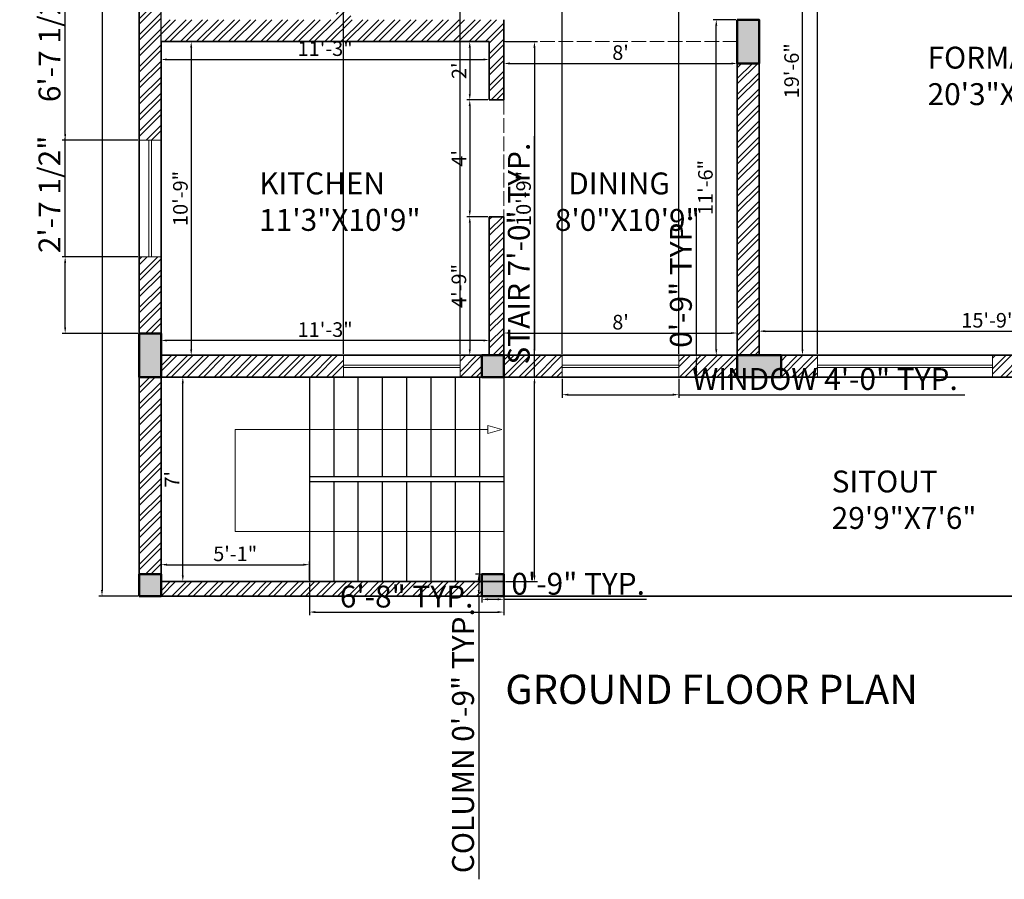
# Model space of a CAD drawing. Units: inches. Extents: x 4153 to 5577, y 785 to 1503.
# Tile 6 of 11: x 4962 to 5367, y 785 to 1138. Entities that reach past the tile are written whole.
import ezdxf

# ---------------------------------------------------------------- set-up
doc = ezdxf.new("R2010")
doc.units = ezdxf.units.IN
doc.linetypes.add('ACAD_ISO02W100', pattern=[15, 12, -3])
for name, color, linetype, lineweight in [('A-ANNO-DIMS', 2, 'Continuous', 18), ('A-ANNO-SYMB', 7, 'Continuous', 18), ('A-ANNO-TEXT', 7, 'Continuous', 35), ('A-AREA-IDEN', 7, 'Continuous', 25), ('A-COLS', 7, 'Continuous', 50), ('A-FLOR-STRS', 7, 'Continuous', 25), ('A-GLAZ', 4, 'Continuous', 18), ('A-WALL', 7, 'Continuous', 35), ('A-WALL-OVHD', 7, 'ACAD_ISO02W100', 18)]:
    doc.layers.add(name, color=color, linetype=linetype, lineweight=lineweight)
doc.layers.add('A-WALL-PATT', color=251, linetype='Continuous', lineweight=13, true_color=0x636466)
doc.styles.get("Standard").update_dxf_attribs({"font": 'arial.ttf'})
doc.dimstyles.new('ISO-25', dxfattribs={"dimtxt": 9, "dimasz": 2.5, "dimexe": 1.25, "dimexo": 0.625, "dimtad": 1, "dimlunit": 3, "dimtxsty": 'Standard', "dimcen": 2.5, "dimadec": 0, "dimazin": 0, "dimtfac": 1, "dimtmove": 0, "dimatfit": 3, "dimfxl": 1, "dimarcsym": 0})

# ---------------------------------------------------------------- blocks, each defined once
blk = doc.blocks.new('*D24')
at = {"layer": 'A-ANNO-DIMS', "color": 0, "lineweight": -2, "transparency": 16777216}
for p, q in [((5010.63, 1444.49), (4994.72, 1444.49)), ((4995.97, 1441.99), (4995.97, 903.99)), ((5010.63, 901.49), (4994.72, 901.49))]:
    blk.add_line(p, q, dxfattribs=at)
at = {"layer": 'A-ANNO-DIMS', "color": 0, "transparency": 16777216}
for points in [[(4995.55, 1441.99), (4996.38, 1441.99), (4995.97, 1444.49)], [(4995.55, 903.99), (4996.38, 903.99), (4995.97, 901.49)]]:
    blk.add_solid(points, dxfattribs=at)
at = {"layer": 'Defpoints', "color": 0, "transparency": 16777216}
for p in [(5011.25, 1444.49), (4995.97, 901.49), (5011.25, 901.49)]:
    blk.add_point(p, dxfattribs=at)
at = {"layer": 'A-ANNO-DIMS', "color": 0, "transparency": 16777216, "insert": (4990.74, 1172.99), "char_height": 9, "attachment_point": 5, "rotation": 90}
blk.add_mtext('45\'-3"', dxfattribs=at)
blk = doc.blocks.new('*D44')
at = {"layer": 'A-ANNO-DIMS', "color": 0, "lineweight": -2, "transparency": 16777216}
for p, q in [((5020.88, 1129.49), (5033.91, 1129.49)), ((5032.66, 1126.99), (5032.66, 1002.99)), ((5020.88, 1000.49), (5033.91, 1000.49))]:
    blk.add_line(p, q, dxfattribs=at)
at = {"layer": 'A-ANNO-DIMS', "color": 0, "transparency": 16777216}
for points in [[(5032.25, 1126.99), (5033.08, 1126.99), (5032.66, 1129.49)], [(5032.25, 1002.99), (5033.08, 1002.99), (5032.66, 1000.49)]]:
    blk.add_solid(points, dxfattribs=at)
at = {"layer": 'Defpoints', "color": 0, "transparency": 16777216}
for p in [(5020.25, 1129.49), (5020.25, 1000.49), (5032.66, 1000.49)]:
    blk.add_point(p, dxfattribs=at)
at = {"layer": 'A-ANNO-DIMS', "color": 0, "transparency": 16777216, "insert": (5028.97, 1064.99), "char_height": 6, "attachment_point": 5, "rotation": 90}
blk.add_mtext('10\'-9"', dxfattribs=at)
blk = doc.blocks.new('*D45')
at = {"layer": 'A-ANNO-DIMS', "color": 0, "lineweight": -2, "transparency": 16777216}
for p, q in [((5020.25, 1128.86), (5020.25, 1120.87)), ((5155.25, 1128.86), (5155.25, 1120.87)), ((5022.75, 1122.12), (5152.75, 1122.12))]:
    blk.add_line(p, q, dxfattribs=at)
at = {"layer": 'A-ANNO-DIMS', "color": 0, "transparency": 16777216}
for points in [[(5022.75, 1122.54), (5022.75, 1121.71), (5020.25, 1122.12)], [(5152.75, 1122.54), (5152.75, 1121.71), (5155.25, 1122.12)]]:
    blk.add_solid(points, dxfattribs=at)
at = {"layer": 'Defpoints', "color": 0, "transparency": 16777216}
for p in [(5020.25, 1129.49), (5155.25, 1129.49), (5155.25, 1122.12)]:
    blk.add_point(p, dxfattribs=at)
at = {"layer": 'A-ANNO-DIMS', "color": 0, "transparency": 16777216, "insert": (5087.75, 1125.81), "char_height": 6, "attachment_point": 5}
blk.add_mtext('11\'-3"', dxfattribs=at)
blk = doc.blocks.new('*D46')
at = {"layer": 'A-ANNO-DIMS', "color": 0, "lineweight": -2, "transparency": 16777216}
for p, q in [((5154.63, 1129.49), (5145.98, 1129.49)), ((5147.23, 1126.99), (5147.23, 1107.99)), ((5154.63, 1105.49), (5145.98, 1105.49))]:
    blk.add_line(p, q, dxfattribs=at)
at = {"layer": 'A-ANNO-DIMS', "color": 0, "transparency": 16777216}
for points in [[(5146.81, 1126.99), (5147.65, 1126.99), (5147.23, 1129.49)], [(5146.81, 1107.99), (5147.65, 1107.99), (5147.23, 1105.49)]]:
    blk.add_solid(points, dxfattribs=at)
at = {"layer": 'Defpoints', "color": 0, "transparency": 16777216}
for p in [(5155.25, 1129.49), (5147.23, 1105.49), (5155.25, 1105.49)]:
    blk.add_point(p, dxfattribs=at)
at = {"layer": 'A-ANNO-DIMS', "color": 0, "transparency": 16777216, "insert": (5143.59, 1117.49), "char_height": 6, "attachment_point": 5, "rotation": 90}
blk.add_mtext("2'", dxfattribs=at)
blk = doc.blocks.new('*D47')
at = {"layer": 'A-ANNO-DIMS', "color": 0, "lineweight": -2, "transparency": 16777216}
for p, q in [((5154.63, 1105.49), (5145.98, 1105.49)), ((5147.23, 1102.99), (5147.23, 1059.99)), ((5154.63, 1057.49), (5145.98, 1057.49))]:
    blk.add_line(p, q, dxfattribs=at)
at = {"layer": 'A-ANNO-DIMS', "color": 0, "transparency": 16777216}
for points in [[(5146.81, 1102.99), (5147.65, 1102.99), (5147.23, 1105.49)], [(5146.81, 1059.99), (5147.65, 1059.99), (5147.23, 1057.49)]]:
    blk.add_solid(points, dxfattribs=at)
at = {"layer": 'Defpoints', "color": 0, "transparency": 16777216}
for p in [(5155.25, 1105.49), (5147.23, 1057.49), (5155.25, 1057.49)]:
    blk.add_point(p, dxfattribs=at)
at = {"layer": 'A-ANNO-DIMS', "color": 0, "transparency": 16777216, "insert": (5143.61, 1081.49), "char_height": 6, "attachment_point": 5, "rotation": 90}
blk.add_mtext("4'", dxfattribs=at)
blk = doc.blocks.new('*D48')
at = {"layer": 'A-ANNO-DIMS', "color": 0, "lineweight": -2, "transparency": 16777216}
for p, q in [((5154.63, 1057.49), (5145.98, 1057.49)), ((5147.23, 1054.99), (5147.23, 1002.99)), ((5154.63, 1000.49), (5145.98, 1000.49))]:
    blk.add_line(p, q, dxfattribs=at)
at = {"layer": 'A-ANNO-DIMS', "color": 0, "transparency": 16777216}
for points in [[(5146.81, 1054.99), (5147.65, 1054.99), (5147.23, 1057.49)], [(5146.81, 1002.99), (5147.65, 1002.99), (5147.23, 1000.49)]]:
    blk.add_solid(points, dxfattribs=at)
at = {"layer": 'Defpoints', "color": 0, "transparency": 16777216}
for p in [(5155.25, 1057.49), (5147.23, 1000.49), (5155.25, 1000.49)]:
    blk.add_point(p, dxfattribs=at)
at = {"layer": 'A-ANNO-DIMS', "color": 0, "transparency": 16777216, "insert": (5143.54, 1028.99), "char_height": 6, "attachment_point": 5, "rotation": 90}
blk.add_mtext('4\'-9"', dxfattribs=at)
blk = doc.blocks.new('*D49')
at = {"layer": 'A-ANNO-DIMS', "color": 0, "lineweight": -2, "transparency": 16777216}
for p, q in [((5020.25, 1001.11), (5020.25, 1007.84)), ((5152.75, 1006.59), (5022.75, 1006.59)), ((5155.25, 1001.11), (5155.25, 1007.84))]:
    blk.add_line(p, q, dxfattribs=at)
at = {"layer": 'A-ANNO-DIMS', "color": 0, "transparency": 16777216}
for points in [[(5022.75, 1007), (5022.75, 1006.17), (5020.25, 1006.59)], [(5152.75, 1007), (5152.75, 1006.17), (5155.25, 1006.59)]]:
    blk.add_solid(points, dxfattribs=at)
at = {"layer": 'Defpoints', "color": 0, "transparency": 16777216}
for p in [(5020.25, 1006.59), (5020.25, 1000.49), (5155.25, 1000.49)]:
    blk.add_point(p, dxfattribs=at)
at = {"layer": 'A-ANNO-DIMS', "color": 0, "transparency": 16777216, "insert": (5087.75, 1010.28), "char_height": 6, "attachment_point": 5}
blk.add_mtext('11\'-3"', dxfattribs=at)
blk = doc.blocks.new('*D50')
at = {"layer": 'A-ANNO-DIMS', "color": 0, "lineweight": -2, "transparency": 16777216}
for p, q in [((5161.25, 1128.86), (5161.25, 1119.24)), ((5257.25, 1128.86), (5257.25, 1119.24)), ((5163.75, 1120.49), (5254.75, 1120.49))]:
    blk.add_line(p, q, dxfattribs=at)
at = {"layer": 'A-ANNO-DIMS', "color": 0, "transparency": 16777216}
for points in [[(5163.75, 1120.91), (5163.75, 1120.07), (5161.25, 1120.49)], [(5254.75, 1120.91), (5254.75, 1120.07), (5257.25, 1120.49)]]:
    blk.add_solid(points, dxfattribs=at)
at = {"layer": 'Defpoints', "color": 0, "transparency": 16777216}
for p in [(5161.25, 1129.49), (5257.25, 1129.49), (5257.25, 1120.49)]:
    blk.add_point(p, dxfattribs=at)
at = {"layer": 'A-ANNO-DIMS', "color": 0, "transparency": 16777216, "insert": (5209.25, 1124.18), "char_height": 6, "attachment_point": 5}
blk.add_mtext("8'", dxfattribs=at)
blk = doc.blocks.new('*D51')
at = {"layer": 'A-ANNO-DIMS', "color": 0, "lineweight": -2, "transparency": 16777216}
for p, q in [((5161.88, 1129.49), (5175.08, 1129.49)), ((5173.83, 1126.99), (5173.83, 1002.99)), ((5161.88, 1000.49), (5175.08, 1000.49))]:
    blk.add_line(p, q, dxfattribs=at)
at = {"layer": 'A-ANNO-DIMS', "color": 0, "transparency": 16777216}
for points in [[(5173.41, 1126.99), (5174.24, 1126.99), (5173.83, 1129.49)], [(5173.41, 1002.99), (5174.24, 1002.99), (5173.83, 1000.49)]]:
    blk.add_solid(points, dxfattribs=at)
at = {"layer": 'Defpoints', "color": 0, "transparency": 16777216}
for p in [(5161.25, 1129.49), (5161.25, 1000.49), (5173.83, 1000.49)]:
    blk.add_point(p, dxfattribs=at)
at = {"layer": 'A-ANNO-DIMS', "color": 0, "transparency": 16777216, "insert": (5170.14, 1064.99), "char_height": 6, "attachment_point": 5, "rotation": 90}
blk.add_mtext('10\'-9"', dxfattribs=at)
blk = doc.blocks.new('*D52')
at = {"layer": 'A-ANNO-DIMS', "color": 0, "lineweight": -2, "transparency": 16777216}
for p, q in [((5161.25, 1001.11), (5161.25, 1010.89)), ((5163.75, 1009.64), (5254.75, 1009.64)), ((5257.25, 1001.11), (5257.25, 1010.89))]:
    blk.add_line(p, q, dxfattribs=at)
at = {"layer": 'A-ANNO-DIMS', "color": 0, "transparency": 16777216}
for points in [[(5163.75, 1010.05), (5163.75, 1009.22), (5161.25, 1009.64)], [(5254.75, 1010.05), (5254.75, 1009.22), (5257.25, 1009.64)]]:
    blk.add_solid(points, dxfattribs=at)
at = {"layer": 'Defpoints', "color": 0, "transparency": 16777216}
for p in [(5257.25, 1009.64), (5161.25, 1000.49), (5257.25, 1000.49)]:
    blk.add_point(p, dxfattribs=at)
at = {"layer": 'A-ANNO-DIMS', "color": 0, "transparency": 16777216, "insert": (5209.25, 1013.33), "char_height": 6, "attachment_point": 5}
blk.add_mtext("8'", dxfattribs=at)
blk = doc.blocks.new('*D53')
at = {"layer": 'A-ANNO-DIMS', "color": 0, "lineweight": -2, "transparency": 16777216}
for p, q in [((5256.63, 1138.49), (5247.37, 1138.49)), ((5248.62, 1002.99), (5248.62, 1135.99)), ((5256.63, 1000.49), (5247.37, 1000.49))]:
    blk.add_line(p, q, dxfattribs=at)
at = {"layer": 'A-ANNO-DIMS', "color": 0, "transparency": 16777216}
for points in [[(5248.2, 1135.99), (5249.04, 1135.99), (5248.62, 1138.49)], [(5248.2, 1002.99), (5249.04, 1002.99), (5248.62, 1000.49)]]:
    blk.add_solid(points, dxfattribs=at)
at = {"layer": 'Defpoints', "color": 0, "transparency": 16777216}
for p in [(5248.62, 1138.49), (5257.25, 1138.49), (5257.25, 1000.49)]:
    blk.add_point(p, dxfattribs=at)
at = {"layer": 'A-ANNO-DIMS', "color": 0, "transparency": 16777216, "insert": (5244.93, 1069.49), "char_height": 6, "attachment_point": 5, "rotation": 90}
blk.add_mtext('11\'-6"', dxfattribs=at)
blk = doc.blocks.new('*D54')
at = {"layer": 'A-ANNO-DIMS', "color": 0, "lineweight": -2, "transparency": 16777216}
for p, q in [((5266.88, 1234.49), (5285.33, 1234.49)), ((5284.08, 1002.99), (5284.08, 1231.99)), ((5266.88, 1000.49), (5285.33, 1000.49))]:
    blk.add_line(p, q, dxfattribs=at)
at = {"layer": 'A-ANNO-DIMS', "color": 0, "transparency": 16777216}
for points in [[(5283.66, 1231.99), (5284.49, 1231.99), (5284.08, 1234.49)], [(5283.66, 1002.99), (5284.49, 1002.99), (5284.08, 1000.49)]]:
    blk.add_solid(points, dxfattribs=at)
at = {"layer": 'Defpoints', "color": 0, "transparency": 16777216}
for p in [(5266.25, 1234.49), (5284.08, 1234.49), (5266.25, 1000.49)]:
    blk.add_point(p, dxfattribs=at)
at = {"layer": 'A-ANNO-DIMS', "color": 0, "transparency": 16777216, "insert": (5280.39, 1117.49), "char_height": 6, "attachment_point": 5, "rotation": 90}
blk.add_mtext('19\'-6"', dxfattribs=at)
blk = doc.blocks.new('*D55')
at = {"layer": 'A-ANNO-DIMS', "color": 0, "lineweight": -2, "transparency": 16777216}
for p, q in [((5266.25, 1001.11), (5266.25, 1011.66)), ((5268.75, 1010.41), (5452.75, 1010.41)), ((5455.25, 1001.11), (5455.25, 1011.66))]:
    blk.add_line(p, q, dxfattribs=at)
at = {"layer": 'A-ANNO-DIMS', "color": 0, "transparency": 16777216}
for points in [[(5268.75, 1010.82), (5268.75, 1009.99), (5266.25, 1010.41)], [(5452.75, 1010.82), (5452.75, 1009.99), (5455.25, 1010.41)]]:
    blk.add_solid(points, dxfattribs=at)
at = {"layer": 'Defpoints', "color": 0, "transparency": 16777216}
for p in [(5455.25, 1010.41), (5266.25, 1000.49), (5455.25, 1000.49)]:
    blk.add_point(p, dxfattribs=at)
at = {"layer": 'A-ANNO-DIMS', "color": 0, "transparency": 16777216, "insert": (5360.75, 1014.1), "char_height": 6, "attachment_point": 5}
blk.add_mtext('15\'-9"', dxfattribs=at)
blk = doc.blocks.new('*D87')
at = {"layer": 'A-ANNO-DIMS', "color": 0, "lineweight": -2, "transparency": 16777216}
for p, q in [((5020.88, 991.49), (5030.45, 991.49)), ((5029.2, 909.99), (5029.2, 988.99)), ((5020.88, 907.49), (5030.45, 907.49))]:
    blk.add_line(p, q, dxfattribs=at)
at = {"layer": 'A-ANNO-DIMS', "color": 0, "transparency": 16777216}
for points in [[(5028.78, 988.99), (5029.61, 988.99), (5029.2, 991.49)], [(5028.78, 909.99), (5029.61, 909.99), (5029.2, 907.49)]]:
    blk.add_solid(points, dxfattribs=at)
at = {"layer": 'Defpoints', "color": 0, "transparency": 16777216}
for p in [(5020.25, 991.49), (5029.2, 991.49), (5020.25, 907.49)]:
    blk.add_point(p, dxfattribs=at)
at = {"layer": 'A-ANNO-DIMS', "color": 0, "transparency": 16777216, "insert": (5025.57, 949.49), "char_height": 6, "attachment_point": 5, "rotation": 90}
blk.add_mtext("7'", dxfattribs=at)
blk = doc.blocks.new('*D88')
at = {"layer": 'A-ANNO-DIMS', "color": 0, "lineweight": -2, "transparency": 16777216}
for p, q in [((5020.25, 908.11), (5020.25, 915.63)), ((5081.25, 908.11), (5081.25, 915.63)), ((5022.75, 914.38), (5078.75, 914.38))]:
    blk.add_line(p, q, dxfattribs=at)
at = {"layer": 'A-ANNO-DIMS', "color": 0, "transparency": 16777216}
for points in [[(5022.75, 914.8), (5022.75, 913.97), (5020.25, 914.38)], [(5078.75, 914.8), (5078.75, 913.97), (5081.25, 914.38)]]:
    blk.add_solid(points, dxfattribs=at)
at = {"layer": 'Defpoints', "color": 0, "transparency": 16777216}
for p in [(5081.25, 914.38), (5020.25, 907.49), (5081.25, 907.49)]:
    blk.add_point(p, dxfattribs=at)
at = {"layer": 'A-ANNO-DIMS', "color": 0, "transparency": 16777216, "insert": (5050.75, 918.07), "char_height": 6, "attachment_point": 5}
blk.add_mtext('5\'-1"', dxfattribs=at)
blk = doc.blocks.new('WINDOW-48IN')
for p, q in [((0, 9), (0, 0)), ((48, 9), (48, 0)), ((0, 5), (48, 5)), ((0, 4), (48, 4))]:
    blk.add_line(p, q)
blk = doc.blocks.new('WINDOW-72IN')
for p, q in [((0, 9), (0, 0)), ((72, 9), (72, 0)), ((0, 5), (72, 5)), ((0, 4), (72, 4))]:
    blk.add_line(p, q)
blk = doc.blocks.new('COL-9X18IN')
at = {"transparency": 33554687}
h = blk.add_hatch(color=256, dxfattribs=at)
h.dxf.hatch_style = 1
h.paths.add_polyline_path([(9, 18), (0, 18), (0, 0), (9, 0)])
blk.add_lwpolyline([(0, 18), (9, 18), (9, 0), (0, 0)], close=True)
blk = doc.blocks.new('COL-9X9IN')
at = {"transparency": 33554687}
h = blk.add_hatch(color=256, dxfattribs=at)
h.dxf.hatch_style = 1
h.paths.add_polyline_path([(9, 0), (9, 9), (0, 9), (0, 0)])
blk.add_lwpolyline([(0, 9), (9, 9), (9, 0), (0, 0)], close=True)
blk = doc.blocks.new('SITOUT-RETURN-STAIR')
at = {"ltscale": 0.5}
for p, q in [((0, 84), (0, 41)), ((10, 84), (10, 43)), ((20, 84), (20, 43)), ((30, 84), (30, 43)), ((40, 84), (40, 43)), ((50, 84), (50, 43)), ((60, 84), (60, 43)), ((70, 84), (70, 43)), ((80, 84), (80, 41))]:
    blk.add_line(p, q, dxfattribs=at)
for p, q in [((80, 43), (0, 43)), ((80, 41), (0, 41)), ((0, 41), (0, 0)), ((10, 41), (10, 0)), ((20, 41), (20, 0)), ((30, 41), (30, 0)), ((40, 41), (40, 0)), ((50, 41), (50, 0)), ((60, 41), (60, 0)), ((70, 41), (70, 0)), ((80, 41), (80, 0))]:
    blk.add_line(p, q)
blk = doc.blocks.new('STAIR-DIRECTION-RETURN')
at = {"ltscale": 0.5}
for p, q in [((103.89, 42), (0, 42)), ((0, 0), (0, 42)), ((110.5, 0), (0, 0))]:
    blk.add_line(p, q, dxfattribs=at)
blk.add_lwpolyline([(109.65, 42), (103.89, 43.63), (103.89, 40.37)], close=True)
blk = doc.blocks.new('*D100')
at = {"layer": 'A-ANNO-DIMS', "color": 0, "lineweight": -2, "transparency": 16777216}
for p, q in [((5151.63, 910.49), (5149.65, 910.49)), ((5150.9, 907.99), (5150.9, 903.99)), ((5151.63, 901.49), (5149.65, 901.49)), ((5150.9, 901.49), (5150.9, 785.01))]:
    blk.add_line(p, q, dxfattribs=at)
at = {"layer": 'A-ANNO-DIMS', "color": 0, "transparency": 16777216}
for points in [[(5150.49, 907.99), (5151.32, 907.99), (5150.9, 910.49)], [(5150.49, 903.99), (5151.32, 903.99), (5150.9, 901.49)]]:
    blk.add_solid(points, dxfattribs=at)
at = {"layer": 'Defpoints', "color": 0, "transparency": 16777216}
for p in [(5152.25, 910.49), (5150.9, 901.49), (5152.25, 901.49)]:
    blk.add_point(p, dxfattribs=at)
at = {"layer": 'A-ANNO-DIMS', "color": 0, "transparency": 16777216, "insert": (5145.62, 842), "char_height": 9, "attachment_point": 5, "rotation": 90}
blk.add_mtext('COLUMN 0\'-9" TYP.', dxfattribs=at)
blk = doc.blocks.new('*D101')
at = {"layer": 'A-ANNO-DIMS', "color": 0, "lineweight": -2, "transparency": 16777216}
for p, q in [((5152.25, 900.86), (5152.25, 898.89)), ((5154.75, 900.14), (5158.75, 900.14)), ((5161.25, 900.86), (5161.25, 898.89)), ((5161.25, 900.14), (5219.86, 900.14))]:
    blk.add_line(p, q, dxfattribs=at)
at = {"layer": 'A-ANNO-DIMS', "color": 0, "transparency": 16777216}
for points in [[(5154.75, 900.56), (5154.75, 899.72), (5152.25, 900.14)], [(5158.75, 900.56), (5158.75, 899.72), (5161.25, 900.14)]]:
    blk.add_solid(points, dxfattribs=at)
at = {"layer": 'Defpoints', "color": 0, "transparency": 16777216}
for p in [(5152.25, 901.49), (5161.25, 901.49), (5161.25, 900.14)]:
    blk.add_point(p, dxfattribs=at)
at = {"layer": 'A-ANNO-DIMS', "color": 0, "transparency": 16777216, "insert": (5191.81, 905.36), "char_height": 9, "attachment_point": 5}
blk.add_mtext('0\'-9" TYP.', dxfattribs=at)
blk = doc.blocks.new('*D102')
at = {"layer": 'A-ANNO-DIMS', "color": 0, "lineweight": -2, "transparency": 16777216}
for p, q in [((5185.25, 990.86), (5185.25, 983.04)), ((5233.25, 990.86), (5233.25, 983.04)), ((5187.75, 984.29), (5230.75, 984.29)), ((5233.25, 984.29), (5350.89, 984.29))]:
    blk.add_line(p, q, dxfattribs=at)
at = {"layer": 'A-ANNO-DIMS', "color": 0, "transparency": 16777216}
for points in [[(5187.75, 984.71), (5187.75, 983.87), (5185.25, 984.29)], [(5230.75, 984.71), (5230.75, 983.87), (5233.25, 984.29)]]:
    blk.add_solid(points, dxfattribs=at)
at = {"layer": 'Defpoints', "color": 0, "transparency": 16777216}
for p in [(5185.25, 991.49), (5233.25, 991.49), (5233.25, 984.29)]:
    blk.add_point(p, dxfattribs=at)
at = {"layer": 'A-ANNO-DIMS', "color": 0, "transparency": 16777216, "insert": (5293.32, 989.57), "char_height": 9, "attachment_point": 5}
blk.add_mtext('WINDOW 4\'-0" TYP.', dxfattribs=at)
blk = doc.blocks.new('*D103')
at = {"layer": 'A-ANNO-DIMS', "color": 0, "lineweight": -2, "transparency": 16777216}
for p, q in [((5240.45, 1000.49), (5240.45, 1059.1)), ((5233.88, 1000.49), (5241.7, 1000.49)), ((5240.45, 993.99), (5240.45, 997.99)), ((5233.88, 991.49), (5241.7, 991.49))]:
    blk.add_line(p, q, dxfattribs=at)
at = {"layer": 'A-ANNO-DIMS', "color": 0, "transparency": 16777216}
for points in [[(5240.04, 997.99), (5240.87, 997.99), (5240.45, 1000.49)], [(5240.04, 993.99), (5240.87, 993.99), (5240.45, 991.49)]]:
    blk.add_solid(points, dxfattribs=at)
at = {"layer": 'Defpoints', "color": 0, "transparency": 16777216}
for p in [(5233.25, 1000.49), (5240.45, 1000.49), (5233.25, 991.49)]:
    blk.add_point(p, dxfattribs=at)
at = {"layer": 'A-ANNO-DIMS', "color": 0, "transparency": 16777216, "insert": (5235.23, 1031.04), "char_height": 9, "attachment_point": 5, "rotation": 90}
blk.add_mtext('0\'-9" TYP.', dxfattribs=at)
blk = doc.blocks.new('*D140')
at = {"layer": 'A-ANNO-DIMS', "color": 0, "lineweight": -2, "transparency": 16777216}
for p, q in [((5173.85, 991.49), (5173.85, 1090.57)), ((5161.88, 991.49), (5175.1, 991.49)), ((5173.85, 909.99), (5173.85, 988.99)), ((5161.88, 907.49), (5175.1, 907.49))]:
    blk.add_line(p, q, dxfattribs=at)
at = {"layer": 'A-ANNO-DIMS', "color": 0, "transparency": 16777216}
for points in [[(5173.44, 988.99), (5174.27, 988.99), (5173.85, 991.49)], [(5173.44, 909.99), (5174.27, 909.99), (5173.85, 907.49)]]:
    blk.add_solid(points, dxfattribs=at)
at = {"layer": 'Defpoints', "color": 0, "transparency": 16777216}
for p in [(5161.25, 991.49), (5173.85, 991.49), (5161.25, 907.49)]:
    blk.add_point(p, dxfattribs=at)
at = {"layer": 'A-ANNO-DIMS', "color": 0, "transparency": 16777216, "insert": (5168.58, 1042.28), "char_height": 9, "attachment_point": 5, "rotation": 90}
blk.add_mtext('STAIR 7\'-0" TYP.', dxfattribs=at)
blk = doc.blocks.new('*D141')
at = {"layer": 'A-ANNO-DIMS', "color": 0, "lineweight": -2, "transparency": 16777216}
for p, q in [((5081.25, 906.86), (5081.25, 893.64)), ((5161.25, 906.86), (5161.25, 893.64)), ((5083.75, 894.89), (5158.75, 894.89))]:
    blk.add_line(p, q, dxfattribs=at)
at = {"layer": 'A-ANNO-DIMS', "color": 0, "transparency": 16777216}
for points in [[(5083.75, 895.31), (5083.75, 894.47), (5081.25, 894.89)], [(5158.75, 895.31), (5158.75, 894.47), (5161.25, 894.89)]]:
    blk.add_solid(points, dxfattribs=at)
at = {"layer": 'Defpoints', "color": 0, "transparency": 16777216}
for p in [(5081.25, 907.49), (5161.25, 907.49), (5161.25, 894.89)]:
    blk.add_point(p, dxfattribs=at)
at = {"layer": 'A-ANNO-DIMS', "color": 0, "transparency": 16777216, "insert": (5121.25, 900.11), "char_height": 9, "attachment_point": 5}
blk.add_mtext('6\'-8" TYP.', dxfattribs=at)
blk = doc.blocks.new('*D150')
at = {"layer": 'A-ANNO-DIMS', "color": 0, "lineweight": -2, "transparency": 16777216}
for p, q in [((4980.8, 1040.99), (4980.8, 1089.79)), ((5010.63, 1040.99), (4979.55, 1040.99)), ((4980.8, 1011.99), (4980.8, 1038.49)), ((5010.63, 1009.49), (4979.55, 1009.49))]:
    blk.add_line(p, q, dxfattribs=at)
at = {"layer": 'A-ANNO-DIMS', "color": 0, "transparency": 16777216}
for points in [[(4980.39, 1038.49), (4981.22, 1038.49), (4980.8, 1040.99)], [(4980.39, 1011.99), (4981.22, 1011.99), (4980.8, 1009.49)]]:
    blk.add_solid(points, dxfattribs=at)
at = {"layer": 'Defpoints', "color": 0, "transparency": 16777216}
for p in [(4980.8, 1040.99), (5011.25, 1040.99), (5011.25, 1009.49)]:
    blk.add_point(p, dxfattribs=at)
at = {"layer": 'A-ANNO-DIMS', "color": 0, "transparency": 16777216, "insert": (4975.53, 1066.64), "char_height": 9, "attachment_point": 5, "rotation": 90}
blk.add_mtext('2\'-7 1/2"', dxfattribs=at)
blk = doc.blocks.new('*D151')
at = {"layer": 'A-ANNO-DIMS', "color": 0, "lineweight": -2, "transparency": 16777216}
for p, q in [((5010.63, 1168.49), (4979.55, 1168.49)), ((4980.8, 1091.49), (4980.8, 1165.99)), ((5010.63, 1088.99), (4979.55, 1088.99))]:
    blk.add_line(p, q, dxfattribs=at)
at = {"layer": 'A-ANNO-DIMS', "color": 0, "transparency": 16777216}
for points in [[(4980.39, 1165.99), (4981.22, 1165.99), (4980.8, 1168.49)], [(4980.39, 1091.49), (4981.22, 1091.49), (4980.8, 1088.99)]]:
    blk.add_solid(points, dxfattribs=at)
at = {"layer": 'Defpoints', "color": 0, "transparency": 16777216}
for p in [(4980.8, 1168.49), (5011.25, 1168.49), (5011.25, 1088.99)]:
    blk.add_point(p, dxfattribs=at)
at = {"layer": 'A-ANNO-DIMS', "color": 0, "transparency": 16777216, "insert": (4975.53, 1128.74), "char_height": 9, "attachment_point": 5, "rotation": 90}
blk.add_mtext('6\'-7 1/2"', dxfattribs=at)
blk = doc.blocks.new('*D156')
at = {"layer": 'A-ANNO-DIMS', "color": 0, "lineweight": -2, "transparency": 16777216}
for p, q in [((5020.25, 1001.11), (5020.25, 1476.19)), ((5022.75, 1474.94), (5092.75, 1474.94)), ((5095.25, 1001.11), (5095.25, 1476.19))]:
    blk.add_line(p, q, dxfattribs=at)
at = {"layer": 'A-ANNO-DIMS', "color": 0, "transparency": 16777216}
for points in [[(5022.75, 1475.36), (5022.75, 1474.52), (5020.25, 1474.94)], [(5092.75, 1475.36), (5092.75, 1474.52), (5095.25, 1474.94)]]:
    blk.add_solid(points, dxfattribs=at)
at = {"layer": 'Defpoints', "color": 0, "transparency": 16777216}
for p in [(5095.25, 1474.94), (5020.25, 1000.49), (5095.25, 1000.49)]:
    blk.add_point(p, dxfattribs=at)
at = {"layer": 'A-ANNO-DIMS', "color": 0, "transparency": 16777216, "insert": (5057.75, 1480.16), "char_height": 9, "attachment_point": 5}
blk.add_mtext('6\'-3"', dxfattribs=at)
blk = doc.blocks.new('*D157')
at = {"layer": 'A-ANNO-DIMS', "color": 0, "lineweight": -2, "transparency": 16777216}
for p, q in [((5143.25, 1001.11), (5143.25, 1476.19)), ((5145.75, 1474.94), (5182.75, 1474.94)), ((5185.25, 1001.11), (5185.25, 1476.19))]:
    blk.add_line(p, q, dxfattribs=at)
at = {"layer": 'A-ANNO-DIMS', "color": 0, "transparency": 16777216}
for points in [[(5145.75, 1475.36), (5145.75, 1474.52), (5143.25, 1474.94)], [(5182.75, 1475.36), (5182.75, 1474.52), (5185.25, 1474.94)]]:
    blk.add_solid(points, dxfattribs=at)
at = {"layer": 'Defpoints', "color": 0, "transparency": 16777216}
for p in [(5185.25, 1474.94), (5143.25, 1000.49), (5185.25, 1000.49)]:
    blk.add_point(p, dxfattribs=at)
at = {"layer": 'A-ANNO-DIMS', "color": 0, "transparency": 16777216, "insert": (5164.25, 1480.16), "char_height": 9, "attachment_point": 5}
blk.add_mtext('3\'-6"', dxfattribs=at)
blk = doc.blocks.new('*D158')
at = {"layer": 'A-ANNO-DIMS', "color": 0, "lineweight": -2, "transparency": 16777216}
for p, q in [((5233.25, 1001.11), (5233.25, 1476.19)), ((5235.75, 1474.94), (5287.75, 1474.94)), ((5290.25, 1001.11), (5290.25, 1476.19))]:
    blk.add_line(p, q, dxfattribs=at)
at = {"layer": 'A-ANNO-DIMS', "color": 0, "transparency": 16777216}
for points in [[(5235.75, 1475.36), (5235.75, 1474.52), (5233.25, 1474.94)], [(5287.75, 1475.36), (5287.75, 1474.52), (5290.25, 1474.94)]]:
    blk.add_solid(points, dxfattribs=at)
at = {"layer": 'Defpoints', "color": 0, "transparency": 16777216}
for p in [(5290.25, 1474.94), (5233.25, 1000.49), (5290.25, 1000.49)]:
    blk.add_point(p, dxfattribs=at)
at = {"layer": 'A-ANNO-DIMS', "color": 0, "transparency": 16777216, "insert": (5261.75, 1480.16), "char_height": 9, "attachment_point": 5}
blk.add_mtext('4\'-9"', dxfattribs=at)

msp = doc.modelspace()

# ---------------------------------------------------------------- hatches: boundary and pattern name
at = {"layer": 'A-WALL-PATT', "transparency": 33554687}
h = msp.add_hatch(dxfattribs=at)
h.set_pattern_fill('ANSI32', color=256, scale=0.49)
h.set_pattern_definition([(45, (816.3263, 0), (-3.300244, 3.300244), []), (45, (818.5265, 0), (-3.300244, 3.300244), [])])
h.paths.add_polyline_path([(5011.254, 1088.988), (5020.254, 1088.988), (5020.254, 1129.488), (5155.254, 1129.488), (5155.254, 1105.488), (5161.254, 1105.488), (5161.254, 1138.488), (5098.254, 1138.488), (5098.254, 1234.488), (5113.254, 1234.488), (5113.254, 1243.488), (5086.254, 1243.488), (5086.254, 1234.488), (5092.254, 1234.488), (5092.254, 1138.488), (5020.254, 1138.488), (5020.254, 1168.488), (5011.254, 1168.488)])
h.paths.add_polyline_path([(5011.254, 1009.488), (5020.254, 1009.488), (5020.254, 1040.988), (5011.254, 1040.988)])
h.paths.add_polyline_path([(5095.254, 991.488), (5095.254, 1000.488), (5020.254, 1000.488), (5020.254, 991.488)])
h.paths.add_polyline_path([(5011.254, 910.488), (5020.254, 910.488), (5020.254, 991.488), (5011.254, 991.488)])
h.paths.add_polyline_path([(5152.254, 901.488), (5152.254, 907.488), (5020.254, 907.488), (5020.254, 901.488)])
h.paths.add_polyline_path([(5161.254, 1057.488), (5155.254, 1057.488), (5155.254, 1000.488), (5161.254, 1000.488)])
h.paths.add_polyline_path([(5143.254, 991.488), (5152.254, 991.488), (5152.254, 1000.488), (5143.254, 1000.488)])
h.paths.add_polyline_path([(5161.254, 1000.488), (5161.254, 991.488), (5185.254, 991.488), (5185.254, 1000.488)])
h.paths.add_polyline_path([(5257.254, 991.488), (5257.254, 1000.488), (5233.254, 1000.488), (5233.254, 991.488)])
h.paths.add_polyline_path([(5266.254, 1120.488), (5257.254, 1120.488), (5257.254, 1000.488), (5266.254, 1000.488)])
h.paths.add_polyline_path([(5290.254, 991.488), (5290.254, 1000.488), (5275.254, 1000.488), (5275.254, 991.488)])
h.paths.add_polyline_path([(5362.254, 1000.488), (5362.254, 991.488), (5455.254, 991.488), (5455.254, 1000.488)])
h.paths.add_polyline_path([(5509.254, 1009.488), (5518.254, 1009.488), (5518.254, 1036.488), (5509.254, 1036.488)])
h.paths.add_polyline_path([(5503.254, 1000.488), (5503.254, 991.488), (5509.254, 991.488), (5509.254, 1000.488)])
h.paths.add_polyline_path([(5518.254, 1132.488), (5509.254, 1132.488), (5509.254, 1108.488), (5518.254, 1108.488)])
h.paths.add_polyline_path([(5509.254, 1204.488), (5518.254, 1204.488), (5518.254, 1225.488), (5509.254, 1225.488)])
h.paths.add_polyline_path([(5467.254, 1234.488), (5467.254, 1243.488), (5377.254, 1243.488), (5377.254, 1265.228), (5377.254, 1381.488), (5467.254, 1381.488), (5467.254, 1393.488), (5461.254, 1393.488), (5461.254, 1387.488), (5377.254, 1387.488), (5377.254, 1435.488), (5368.254, 1435.488), (5368.254, 1354.488), (5347.254, 1354.488), (5347.254, 1348.488), (5368.254, 1348.488), (5368.254, 1309.488), (5302.254, 1309.488), (5302.254, 1234.488), (5321.754, 1234.488), (5321.754, 1243.488), (5311.254, 1243.488), (5311.254, 1303.488), (5368.254, 1303.488), (5368.254, 1243.488), (5357.754, 1243.488), (5357.754, 1234.488)])
h.paths.add_polyline_path([(5509.254, 1357.488), (5518.254, 1357.488), (5518.254, 1426.488), (5509.254, 1426.488)])
h.paths.add_polyline_path([(5509.254, 1243.488), (5518.254, 1243.488), (5518.254, 1309.488), (5509.254, 1309.488)])
h.paths.add_polyline_path([(5509.254, 1435.488), (5509.254, 1444.488), (5425.254, 1444.488), (5425.254, 1435.488), (5461.254, 1435.488), (5461.254, 1423.488), (5467.254, 1423.488), (5467.254, 1435.488)])
h.paths.add_polyline_path([(5302.254, 1435.488), (5302.254, 1348.488), (5317.254, 1348.488), (5317.254, 1354.488), (5311.254, 1354.488), (5311.254, 1435.488), (5314.254, 1435.488), (5314.254, 1444.488), (5296.254, 1444.488), (5296.254, 1435.488)])
h.paths.add_polyline_path([(5368.254, 1444.488), (5362.254, 1444.488), (5362.254, 1435.488), (5368.254, 1435.488)])
h.paths.add_polyline_path([(5389.254, 1444.488), (5386.254, 1444.488), (5386.254, 1435.488), (5389.254, 1435.488)])
h.paths.add_polyline_path([(5248.254, 1435.488), (5248.254, 1444.488), (5173.254, 1444.488), (5173.254, 1435.488)])
h.paths.add_polyline_path([(5101.254, 1435.488), (5101.254, 1444.488), (5020.254, 1444.488), (5020.254, 1435.488)])
h.paths.add_polyline_path([(5011.254, 1293.488), (5020.254, 1293.488), (5020.254, 1295.242), (5020.254, 1426.488), (5011.254, 1426.488)])
h.paths.add_polyline_path([(5155.254, 1243.488), (5149.254, 1243.488), (5149.254, 1234.488), (5248.254, 1234.488), (5248.254, 1243.488), (5164.254, 1243.488), (5164.254, 1435.488), (5155.254, 1435.488)])
h.paths.add_polyline_path([(5020.254, 1243.488), (5020.254, 1234.488), (5056.254, 1234.488), (5056.254, 1243.488)], flags=17)
h.paths.add_polyline_path([(5020.254, 1225.488), (5011.254, 1225.488), (5011.254, 1198.488), (5020.254, 1198.488)], flags=17)

# ---------------------------------------------------------------- linework, layer by layer
at = {"layer": 'A-WALL'}
for p, q in [((5011.254, 901.488), (5011.254, 1444.488)), ((5161.254, 1105.488), (5161.254, 1138.488)), ((5257.254, 1000.488), (5257.254, 1138.488)), ((5266.254, 1000.488), (5266.254, 1138.488)), ((5020.254, 1129.488), (5155.254, 1129.488)), ((5020.254, 1000.488), (5020.254, 1129.488)), ((5155.254, 1105.488), (5155.254, 1129.488)), ((5155.254, 1105.488), (5161.254, 1105.488)), ((5155.254, 1000.488), (5155.254, 1057.488)), ((5155.254, 1057.488), (5161.254, 1057.488)), ((5161.254, 1000.488), (5161.254, 1057.488)), ((5020.254, 1000.488), (5155.254, 1000.488)), ((5161.254, 1000.488), (5257.254, 1000.488)), ((5266.254, 1000.488), (5455.254, 1000.488)), ((5020.254, 991.488), (5455.254, 991.488)), ((5020.254, 907.488), (5020.254, 991.488)), ((5161.254, 907.488), (5020.254, 907.488)), ((5518.254, 901.488), (5011.254, 901.488))]:
    msp.add_line(p, q, dxfattribs=at)
at = {"layer": 'A-WALL-OVHD', "ltscale": 0.5}
for p, q in [((5161.254, 1129.488), (5257.254, 1129.488)), ((5161.254, 1105.488), (5161.254, 1057.488))]:
    msp.add_line(p, q, dxfattribs=at)

# ---------------------------------------------------------------- block references
at = {"layer": 'A-ANNO-SYMB'}
msp.add_blockref('STAIR-DIRECTION-RETURN', (5050.754, 927.988), dxfattribs=at)
at = {"layer": 'A-COLS'}
for p in [(5257.254, 1120.488), (5011.254, 991.488)]:
    msp.add_blockref('COL-9X18IN', p, dxfattribs=at)
for name, p, rotation in [('COL-9X9IN', (5152.254, 1000.488), 270.0000000000087), ('COL-9X18IN', (5257.254, 1000.488), 270.0000000000049), ('COL-9X9IN', (5011.254, 910.488), 270.0000000000065), ('COL-9X9IN', (5152.254, 910.488), 270.0000000000058)]:
    msp.add_blockref(name, p, dxfattribs=dict(at, rotation=rotation))
at = {"layer": 'A-FLOR-STRS'}
msp.add_blockref('SITOUT-RETURN-STAIR', (5081.254, 907.488), dxfattribs=at)
at = {"layer": 'A-GLAZ', "rotation": 269.9999999999995}
msp.add_blockref('WINDOW-48IN', (5011.254, 1088.988), dxfattribs=at)
at = {"layer": 'A-GLAZ'}
for name, p in [('WINDOW-48IN', (5095.254, 991.488)), ('WINDOW-48IN', (5185.254, 991.488)), ('WINDOW-72IN', (5290.254, 991.488))]:
    msp.add_blockref(name, p, dxfattribs=at)

# ---------------------------------------------------------------- texts
at = {"layer": 'A-ANNO-TEXT', "insert": (5161.858, 869.133), "char_height": 12, "attachment_point": 1}
msp.add_mtext_dynamic_manual_height_columns('{\\fTimes New Roman|b0|i0|c0|p18;GROUND FLOOR PLAN}', width=197.6934, gutter_width=12.5, heights=[0], dxfattribs=at)
at = {"layer": 'A-AREA-IDEN', "char_height": 9, "attachment_point": 1}
for s, width, insert in [('{\\fTimes New Roman|b0|i0|c0|p18;FORMAL LIVING\\P20\'3"X19\'6"}', 119.83324, (5335.538, 1127.378)), ('{\\fTimes New Roman|b0|i0|c0|p18;KITCHEN\\P11\'3"X10\'9"}', 67.35079, (5060.618, 1075.66)), ('{\\fTimes New Roman|b0|i0|c0|p18;  DINING\\P8\'0"X10\'9"}', 67.35079, (5182.226, 1075.66)), ('{\\fTimes New Roman|b0|i0|c0|p18;SITOUT\\P29\'9"X7\'6"}', 119.83324, (5296.095, 953.097))]:
    msp.add_mtext_dynamic_manual_height_columns(s, width=width, gutter_width=12.5, heights=[0], dxfattribs=dict(at, insert=insert))

# ---------------------------------------------------------------- dimensions: what is measured, and where the dimension line sits
at = {"layer": 'A-ANNO-DIMS'}
for base, p1, p2, override, picture, middle in [((5095.254, 1474.938), (5020.254, 1000.488), (5095.254, 1000.488), {"dimdec": 1, "dimlfac": 1, "dimrnd": 0, "dimzin": 1, "dimdsep": 46, "dimlunit": 4, "dimfrac": 2}, '*D156', (5057.754, 1480.162)), ((5185.254, 1474.938), (5143.254, 1000.488), (5185.254, 1000.488), {"dimdec": 1, "dimlfac": 1, "dimrnd": 0, "dimzin": 1, "dimdsep": 46, "dimlunit": 4, "dimfrac": 2}, '*D157', (5164.254, 1480.162)), ((5290.254, 1474.938), (5233.254, 1000.488), (5290.254, 1000.488), {"dimdec": 1, "dimlfac": 1, "dimrnd": 0, "dimzin": 1, "dimdsep": 46, "dimlunit": 4, "dimfrac": 2}, '*D158', (5261.754, 1480.159)), ((5155.254, 1122.123), (5020.254, 1129.488), (5155.254, 1129.488), {"dimtxt": 6, "dimclrd": 0, "dimclre": 0, "dimclrt": 0}, '*D45', (5087.754, 1125.814)), ((5257.254, 1120.488), (5161.254, 1129.488), (5257.254, 1129.488), {"dimtxt": 6, "dimclrd": 0, "dimclre": 0, "dimclrt": 0}, '*D50', (5209.254, 1124.177)), ((5257.254, 1009.638), (5161.254, 1000.488), (5257.254, 1000.488), {"dimtxt": 6, "dimclrd": 0, "dimclre": 0, "dimclrt": 0}, '*D52', (5209.254, 1013.326)), ((5455.254, 1010.407), (5266.254, 1000.488), (5455.254, 1000.488), {"dimtxt": 6, "dimclrd": 0, "dimclre": 0, "dimclrt": 0}, '*D55', (5360.754, 1014.095)), ((5020.254, 1006.587), (5155.254, 1000.488), (5020.254, 1000.488), {"dimtxt": 6, "dimclrd": 0, "dimclre": 0, "dimclrt": 0}, '*D49', (5087.754, 1010.278)), ((5081.254, 914.383), (5020.254, 907.488), (5081.254, 907.488), {"dimtxt": 6, "dimclrd": 0, "dimclre": 0, "dimclrt": 0}, '*D88', (5050.754, 918.071))]:
    dim = msp.add_linear_dim(base=base, p1=p1, p2=p2, dimstyle='ISO-25', override=override, dxfattribs=at)
    dim.commit()
    dim.dimension.update_dxf_attribs({"geometry": picture, "text_midpoint": middle})
for base, p1, p2, override, picture, middle in [((4995.968, 901.488), (5011.254, 1444.488), (5011.254, 901.488), {"dimclrd": 0, "dimclre": 0, "dimclrt": 0}, '*D24', (4990.745, 1172.988)), ((5284.077, 1234.488), (5266.254, 1000.488), (5266.254, 1234.488), {"dimtxt": 6, "dimclrd": 0, "dimclre": 0, "dimclrt": 0}, '*D54', (5280.389, 1117.488)), ((4980.804, 1168.488), (5011.254, 1088.988), (5011.254, 1168.488), {"dimdec": 1, "dimlfac": 1, "dimrnd": 0, "dimzin": 1, "dimdsep": 46, "dimlunit": 4, "dimfrac": 2}, '*D151', (4975.525, 1128.738)), ((5248.621, 1138.488), (5257.254, 1000.488), (5257.254, 1138.488), {"dimtxt": 6, "dimclrd": 0, "dimclre": 0, "dimclrt": 0}, '*D53', (5244.932, 1069.488)), ((5032.663, 1000.488), (5020.254, 1129.488), (5020.254, 1000.488), {"dimtxt": 6, "dimclrd": 0, "dimclre": 0, "dimclrt": 0}, '*D44', (5028.974, 1064.988)), ((5147.231, 1105.488), (5155.254, 1129.488), (5155.254, 1105.488), {"dimtxt": 6, "dimclrd": 0, "dimclre": 0, "dimclrt": 0}, '*D46', (5143.593, 1117.488)), ((5173.825, 1000.488), (5161.254, 1129.488), (5161.254, 1000.488), {"dimtxt": 6, "dimclrd": 0, "dimclre": 0, "dimclrt": 0}, '*D51', (5170.137, 1064.988)), ((5147.231, 1057.488), (5155.254, 1105.488), (5155.254, 1057.488), {"dimtxt": 6, "dimclrd": 0, "dimclre": 0, "dimclrt": 0, "dimtmove": 1}, '*D47', (5143.606, 1081.488)), ((4980.804, 1040.988), (5011.254, 1009.488), (5011.254, 1040.988), {"dimdec": 1, "dimlfac": 1, "dimrnd": 0, "dimzin": 1, "dimdsep": 46, "dimlunit": 4, "dimfrac": 2}, '*D150', (4975.525, 1066.638)), ((5147.231, 1000.488), (5155.254, 1057.488), (5155.254, 1000.488), {"dimtxt": 6, "dimclrd": 0, "dimclre": 0, "dimclrt": 0, "dimtmove": 1}, '*D48', (5143.542, 1028.988)), ((5029.198, 991.488), (5020.254, 907.488), (5020.254, 991.488), {"dimtxt": 6, "dimclrd": 0, "dimclre": 0, "dimclrt": 0}, '*D87', (5025.573, 949.488))]:
    dim = msp.add_linear_dim(base=base, p1=p1, p2=p2, angle=90, dimstyle='ISO-25', override=override, dxfattribs=at)
    dim.commit()
    dim.dimension.update_dxf_attribs({"geometry": picture, "text_midpoint": middle})
for base, p1, p2, angle, text, picture, middle in [((5173.854, 991.488), (5161.254, 907.488), (5161.254, 991.488), 90, 'STAIR <> TYP.', '*D140', (5168.575, 1042.281)), ((5240.454, 1000.488), (5233.254, 991.488), (5233.254, 1000.488), 90, '<> TYP.', '*D103', (5235.234, 1031.043)), ((5161.254, 900.138), (5152.254, 901.488), (5161.254, 901.488), 0, '<> TYP.', '*D101', (5191.809, 905.359)), ((5150.904, 901.488), (5152.254, 910.488), (5152.254, 901.488), 270, 'COLUMN <> TYP.', '*D100', (5145.622, 841.997))]:
    dim = msp.add_linear_dim(base=base, p1=p1, p2=p2, angle=angle, text=text, dimstyle='ISO-25', override={"dimdec": 1, "dimlfac": 1, "dimrnd": 0, "dimzin": 1, "dimdsep": 46, "dimlunit": 4, "dimfrac": 2}, dxfattribs=at)
    dim.commit()
    dim.dimension.update_dxf_attribs({"geometry": picture, "text_midpoint": middle})
for base, p1, p2, text, picture, middle in [((5233.254, 984.288), (5185.254, 991.488), (5233.254, 991.488), 'WINDOW <> TYP.', '*D102', (5293.323, 989.57)), ((5161.254, 894.888), (5081.254, 907.488), (5161.254, 907.488), '<> TYP.', '*D141', (5121.254, 900.109))]:
    dim = msp.add_linear_dim(base=base, p1=p1, p2=p2, text=text, dimstyle='ISO-25', override={"dimdec": 1, "dimlfac": 1, "dimrnd": 0, "dimzin": 1, "dimdsep": 46, "dimlunit": 4, "dimfrac": 2}, dxfattribs=at)
    dim.commit()
    dim.dimension.update_dxf_attribs({"geometry": picture, "text_midpoint": middle})

doc.saveas('drawing.dxf')
